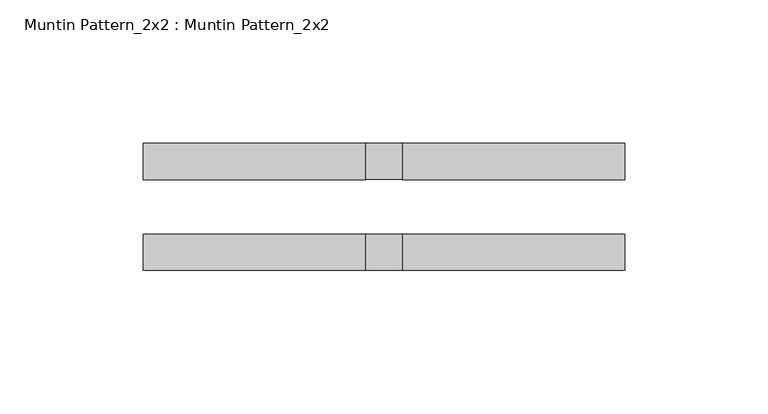
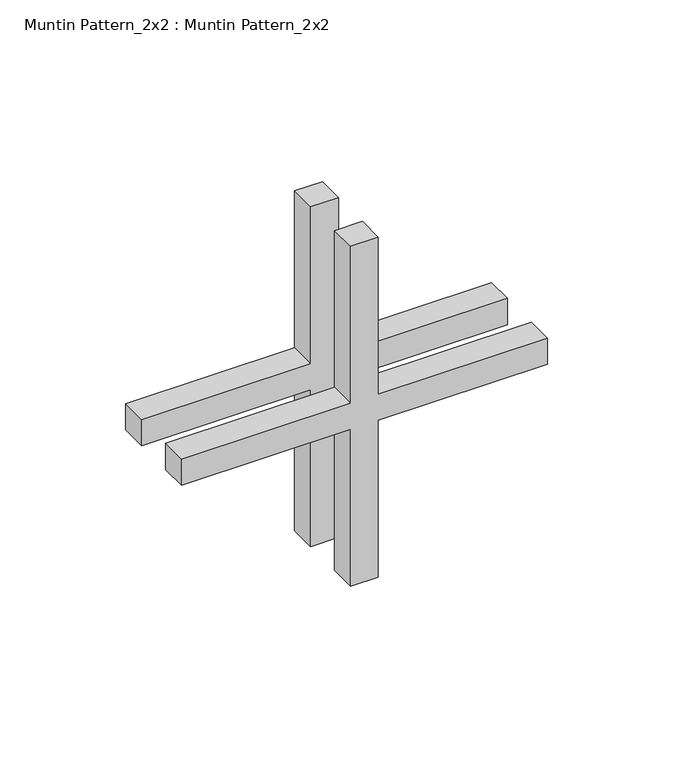
"""IFC4 building model written with IfcOpenShell, lengths in millimetres: proxy geometry, Muntin Pattern_2x2 : Muntin Pattern_2x2."""

from ifc_helpers import new_model, si_unit, frame, origin, place, context, project, spatial, polyline, outline, extrude, source, transform, mapped, element, save


def muntin_pattern_2x2_muntin_pattern_2x2_7edc5815(model_context):
    return source(origin(), model_context, "Body", "SweptSolid", [
        extrude(outline(polyline([(88.9, -6.35), (88.9, -84.1375), (76.2, -84.1375), (76.2, -6.35), (0.0, -6.35), (0.0, 6.35), (76.2, 6.35), (76.2, 84.1375), (88.9, 84.1375), (88.9, 6.35), (165.1, 6.35), (165.1, -6.35), (88.9, -6.35)])), frame((0.0, -22.225, 0.0), z_axis=(0.0, 1.0, 0.0), x_axis=(0.0, 0.0, 1.0)), (0.0, 0.0, 1.0), 12.7),
        extrude(outline(polyline([(88.9, -6.35), (88.9, -84.1375), (76.2, -84.1375), (76.2, -6.35), (0.0, -6.35), (0.0, 6.35), (76.2, 6.35), (76.2, 84.1375), (88.9, 84.1375), (88.9, 6.35), (165.1, 6.35), (165.1, -6.35), (88.9, -6.35)])), frame((0.0, 9.525, 0.0), z_axis=(0.0, 1.0, 0.0), x_axis=(0.0, 0.0, 1.0)), (0.0, 0.0, 1.0), 12.7),
    ])


if __name__ == "__main__":
    model = new_model("IFC4")
    model_context = context("Model", 3, world=origin())
    ifc_project = project(units=[si_unit("LENGTHUNIT", "METRE", prefix="MILLI")], contexts=[model_context])
    site = spatial("IfcSite", under=ifc_project)
    building = spatial("IfcBuilding", under=site)
    placement = place(None, origin())
    muntin_pattern_2x2_muntin_pattern_2x2_shape = muntin_pattern_2x2_muntin_pattern_2x2_7edc5815(model_context)
    element("IfcBuildingElementProxy", 1, Name="Muntin Pattern_2x2 : Muntin Pattern_2x2", ObjectType="Muntin Pattern_2x2 : Muntin Pattern_2x2", at=placement, inside=building, context=model_context, shape_type="MappedRepresentation", body=[
        mapped(muntin_pattern_2x2_muntin_pattern_2x2_shape, transform((0.0, 0.0, 0.0), x_axis=(1.0, 0.0, 0.0), y_axis=(0.0, 1.0, 0.0), z_axis=(0.0, 0.0, 1.0))),
    ])
    save(model, "model.ifc")

# Revit data of these elements
# Type "Muntin Pattern_2x2 : Muntin Pattern_2x2"
#   Width [instance default] = 4' - 0"
#   Thickness = 0' - 0 1/2"
#   Height [instance default] = 4' - 0"
#   Distance = 0' - 0 3/4"
#   Interior Material [instance default] = none
#   Exterior Material [instance default] = none
#   Default Elevation = 0
# Element 1 (IfcBuildingElementProxy, "Muntin Pattern_2x2 : Muntin Pattern_2x2")
#   Width = 0' - 6 5/8"
#   Height = 0' - 6 1/2"
#   Interior Material = Wood - Stained
#   Exterior Material = Clad - White
#   Materials on its faces: "Clad - White", "Wood - Stained"
# Materials
#   "Clad - White": class "Wood", colour RGB 242 242 238, transparency 0, Cost = 0
#   "Wood - Stained": class "Wood", colour RGB 224 178 126, transparency 0, Cost = 0
